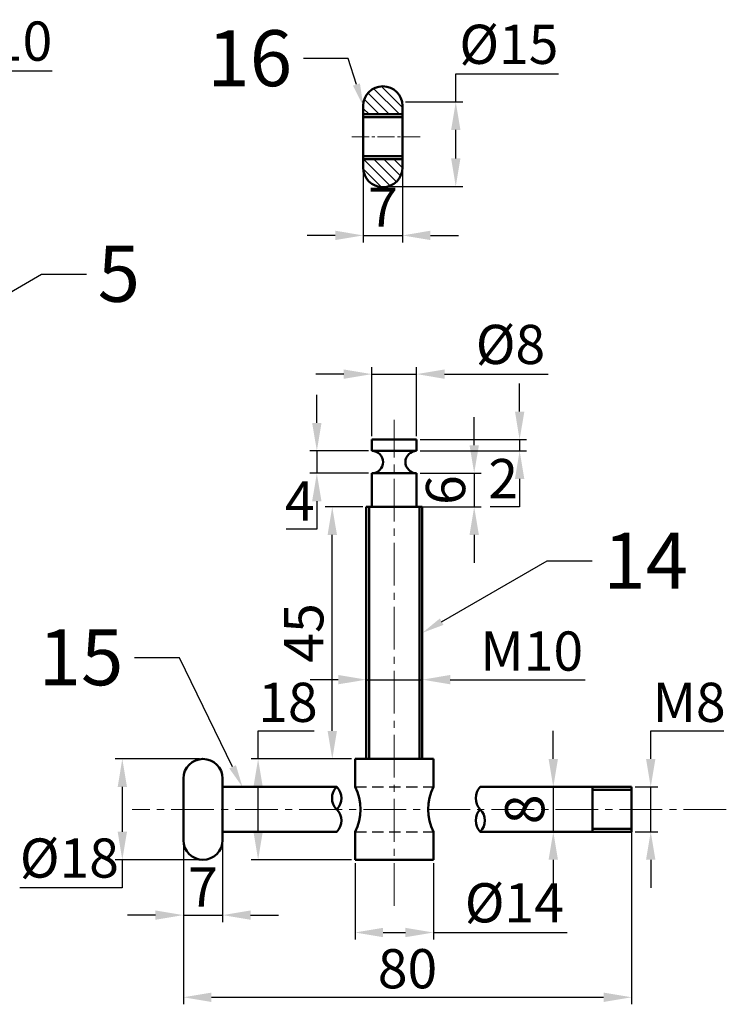
# Model space of a CAD drawing. Units: millimetres. Extents: x 434 to 1535, y -197 to 318.
# Tile 6 of 9: x 920 to 1046, y -7 to 168. Entities that reach past the tile are written whole.
import ezdxf
from ezdxf import colors
from ezdxf.entities.mleader import LeaderData, LeaderLine
from ezdxf.math import Vec2, Vec3

# ---------------------------------------------------------------- set-up
doc = ezdxf.new("R2010")
doc.units = ezdxf.units.MM
doc.header["$LTSCALE"] = 0.4
doc.linetypes.add('CENTER2', pattern=[28.575, 19.05, -3.175, 3.175, -3.175])
doc.linetypes.add('DASHED', pattern=[19.05, 12.7, -6.35])
for name, color, linetype, lineweight in [('M-CNTR', 1, 'CENTER2', 18), ('M-DIMS', 2, 'Continuous', 25), ('M-HATC', 8, 'Continuous', 18), ('M-HIDN', 6, 'DASHED', 25), ('M-OUTL', 7, 'Continuous', 50), ('M-TEXT', 3, 'Continuous', 25)]:
    doc.layers.add(name, color=color, linetype=linetype, lineweight=lineweight)
doc.styles.get("Standard").update_dxf_attribs({"font": 'arial.ttf'})
doc.dimstyles.new('ISO-25', dxfattribs={"dimtxt": 7, "dimasz": 5, "dimexe": 1.25, "dimexo": 0.625, "dimtad": 1, "dimtoh": 1, "dimdec": 0, "dimtxsty": 'Standard', "dimcen": 2.5, "dimadec": 0, "dimazin": 0, "dimtfac": 1, "dimtdec": 0, "dimtmove": 0, "dimatfit": 3, "dimfxl": 1, "dimarcsym": 0})

# ---------------------------------------------------------------- blocks, each defined once
blk = doc.blocks.new('*D61')
at = {"layer": 'Defpoints', "color": 0, "ltscale": 0.4, "transparency": 16777216}
for p in [(901.74, 149.22), (901.74, 139.22), (907.09, 139.22)]:
    blk.add_point(p, dxfattribs=at)
at = {"layer": 'M-DIMS', "color": 0, "lineweight": -2, "ltscale": 0.4, "transparency": 16777216}
for p, q in [((907.09, 154.22), (907.09, 159.22)), ((907.09, 159.22), (925.34, 159.22)), ((902.36, 149.22), (908.34, 149.22)), ((907.09, 139.22), (907.09, 149.22)), ((902.36, 139.22), (908.34, 139.22)), ((907.09, 134.22), (907.09, 129.22))]:
    blk.add_line(p, q, dxfattribs=at)
at = {"layer": 'M-DIMS', "color": 0, "ltscale": 0.4, "transparency": 16777216}
for points in [[(906.26, 154.22), (907.93, 154.22), (907.09, 149.22)], [(906.26, 134.22), (907.93, 134.22), (907.09, 139.22)]]:
    blk.add_solid(points, dxfattribs=at)
at = {"layer": 'M-DIMS', "color": 0, "ltscale": 0.4, "transparency": 16777216, "insert": (916.53, 163.61), "char_height": 7, "attachment_point": 5}
blk.add_mtext('%%C10', dxfattribs=at)
blk = doc.blocks.new('*U76')
at = {"layer": 'M-CNTR', "color": 0, "transparency": 16777216}
blk.add_line((0, -17.2), (0, 69.52), dxfattribs=at)
blk = doc.blocks.new('*U77')
at = {"layer": 'M-CNTR', "color": 0, "transparency": 16777216}
blk.add_line((59.26, 0), (-46.77, 0), dxfattribs=at)
blk = doc.blocks.new('*D78')
at = {"layer": 'Defpoints', "color": 0, "ltscale": 0.4, "transparency": 16777216}
for p in [(979.4, 18.37), (993.4, 18.37), (993.4, 5.38)]:
    blk.add_point(p, dxfattribs=at)
at = {"layer": 'M-DIMS', "color": 0, "lineweight": -2, "ltscale": 0.4, "transparency": 16777216}
for p, q in [((979.4, 17.75), (979.4, 4.13)), ((993.4, 17.75), (993.4, 4.13)), ((984.4, 5.38), (988.4, 5.38)), ((993.4, 5.38), (1017.27, 5.38))]:
    blk.add_line(p, q, dxfattribs=at)
at = {"layer": 'M-DIMS', "color": 0, "ltscale": 0.4, "transparency": 16777216}
for points in [[(984.4, 6.22), (984.4, 4.55), (979.4, 5.38)], [(988.4, 6.22), (988.4, 4.55), (993.4, 5.38)]]:
    blk.add_solid(points, dxfattribs=at)
at = {"layer": 'M-DIMS', "color": 0, "ltscale": 0.4, "transparency": 16777216, "insert": (1007.83, 9.78), "char_height": 7, "attachment_point": 5}
blk.add_mtext('%%C14', dxfattribs=at)
blk = doc.blocks.new('*D79')
at = {"layer": 'Defpoints', "color": 0, "ltscale": 0.4, "transparency": 16777216}
for p in [(948.77, 27.37), (1028.77, 27.37), (1028.77, -6.18)]:
    blk.add_point(p, dxfattribs=at)
at = {"layer": 'M-DIMS', "color": 0, "lineweight": -2, "ltscale": 0.4, "transparency": 16777216}
for p, q in [((948.77, 26.75), (948.77, -7.43)), ((1028.77, 26.75), (1028.77, -7.43)), ((953.77, -6.18), (1023.77, -6.18))]:
    blk.add_line(p, q, dxfattribs=at)
at = {"layer": 'M-DIMS', "color": 0, "ltscale": 0.4, "transparency": 16777216}
for points in [[(953.77, -5.35), (953.77, -7.02), (948.77, -6.18)], [(1023.77, -5.35), (1023.77, -7.02), (1028.77, -6.18)]]:
    blk.add_solid(points, dxfattribs=at)
at = {"layer": 'M-DIMS', "color": 0, "ltscale": 0.4, "transparency": 16777216, "insert": (988.77, -1.99), "char_height": 7, "attachment_point": 5}
blk.add_mtext('80', dxfattribs=at)
blk = doc.blocks.new('*D82')
at = {"layer": 'Defpoints', "color": 0, "ltscale": 0.4, "transparency": 16777216}
for p in [(1028.77, 31.37), (1028.77, 23.37), (1032.18, 23.37)]:
    blk.add_point(p, dxfattribs=at)
at = {"layer": 'M-DIMS', "color": 0, "lineweight": -2, "ltscale": 0.4, "transparency": 16777216}
for p, q in [((1032.18, 36.37), (1032.18, 41.37)), ((1032.18, 41.37), (1045.23, 41.37)), ((1029.4, 31.37), (1033.43, 31.37)), ((1032.18, 23.37), (1032.18, 31.37)), ((1029.4, 23.37), (1033.43, 23.37)), ((1032.18, 18.37), (1032.18, 13.37))]:
    blk.add_line(p, q, dxfattribs=at)
at = {"layer": 'M-DIMS', "color": 0, "ltscale": 0.4, "transparency": 16777216}
for points in [[(1031.34, 36.37), (1033.01, 36.37), (1032.18, 31.37)], [(1031.34, 18.37), (1033.01, 18.37), (1032.18, 23.37)]]:
    blk.add_solid(points, dxfattribs=at)
at = {"layer": 'M-DIMS', "color": 0, "ltscale": 0.4, "transparency": 16777216, "insert": (1039.02, 45.57), "char_height": 7, "attachment_point": 5}
blk.add_mtext('M8', dxfattribs=at)
blk = doc.blocks.new('*D83')
at = {"layer": 'Defpoints', "color": 0, "ltscale": 0.4, "transparency": 16777216}
for p in [(952.27, 36.37), (937.87, 18.37), (952.27, 18.37)]:
    blk.add_point(p, dxfattribs=at)
at = {"layer": 'M-DIMS', "color": 0, "lineweight": -2, "ltscale": 0.4, "transparency": 16777216}
for p, q in [((951.65, 36.37), (936.62, 36.37)), ((937.87, 31.37), (937.87, 23.37)), ((951.65, 18.37), (936.62, 18.37)), ((937.87, 18.37), (937.87, 13.37)), ((937.87, 13.37), (919.59, 13.37))]:
    blk.add_line(p, q, dxfattribs=at)
at = {"layer": 'M-DIMS', "color": 0, "ltscale": 0.4, "transparency": 16777216}
for points in [[(937.04, 31.37), (938.71, 31.37), (937.87, 36.37)], [(937.04, 23.37), (938.71, 23.37), (937.87, 18.37)]]:
    blk.add_solid(points, dxfattribs=at)
at = {"layer": 'M-DIMS', "color": 0, "ltscale": 0.4, "transparency": 16777216, "insert": (928.42, 17.77), "char_height": 7, "attachment_point": 5}
blk.add_mtext('%%C18', dxfattribs=at)
blk = doc.blocks.new('*D84')
at = {"layer": 'Defpoints', "color": 0, "ltscale": 0.4, "transparency": 16777216}
for p in [(948.77, 27.37), (955.77, 27.37), (955.77, 8.49)]:
    blk.add_point(p, dxfattribs=at)
at = {"layer": 'M-DIMS', "color": 0, "lineweight": -2, "ltscale": 0.4, "transparency": 16777216}
for p, q in [((948.77, 26.75), (948.77, 7.24)), ((955.77, 26.75), (955.77, 7.24)), ((943.77, 8.49), (938.77, 8.49)), ((948.77, 8.49), (955.77, 8.49)), ((960.77, 8.49), (965.77, 8.49))]:
    blk.add_line(p, q, dxfattribs=at)
at = {"layer": 'M-DIMS', "color": 0, "ltscale": 0.4, "transparency": 16777216}
for points in [[(943.77, 9.32), (943.77, 7.66), (948.77, 8.49)], [(960.77, 9.32), (960.77, 7.66), (955.77, 8.49)]]:
    blk.add_solid(points, dxfattribs=at)
at = {"layer": 'M-DIMS', "color": 0, "ltscale": 0.4, "transparency": 16777216, "insert": (952.27, 12.61), "char_height": 7, "attachment_point": 5}
blk.add_mtext('7', dxfattribs=at)
blk = doc.blocks.new('*D85')
at = {"layer": 'Defpoints', "color": 0, "ltscale": 0.4, "transparency": 16777216}
for p in [(962.11, 36.37), (979.4, 36.37), (979.4, 18.37)]:
    blk.add_point(p, dxfattribs=at)
at = {"layer": 'M-DIMS', "color": 0, "lineweight": -2, "ltscale": 0.4, "transparency": 16777216}
for p, q in [((962.11, 36.37), (962.11, 41.37)), ((962.11, 41.37), (972.12, 41.37)), ((978.78, 36.37), (960.86, 36.37)), ((962.11, 23.37), (962.11, 31.37)), ((978.78, 18.37), (960.86, 18.37))]:
    blk.add_line(p, q, dxfattribs=at)
at = {"layer": 'M-DIMS', "color": 0, "ltscale": 0.4, "transparency": 16777216}
for points in [[(961.28, 31.37), (962.94, 31.37), (962.11, 36.37)], [(961.28, 23.37), (962.94, 23.37), (962.11, 18.37)]]:
    blk.add_solid(points, dxfattribs=at)
at = {"layer": 'M-DIMS', "color": 0, "ltscale": 0.4, "transparency": 16777216, "insert": (967.43, 45.57), "char_height": 7, "attachment_point": 5}
blk.add_mtext('18', dxfattribs=at)
blk = doc.blocks.new('*D86')
at = {"layer": 'Defpoints', "color": 0, "ltscale": 0.4, "transparency": 16777216}
for p in [(975.34, 81.37), (981.4, 81.37), (979.4, 36.37)]:
    blk.add_point(p, dxfattribs=at)
at = {"layer": 'M-DIMS', "color": 0, "lineweight": -2, "ltscale": 0.4, "transparency": 16777216}
for p, q in [((980.78, 81.37), (974.09, 81.37)), ((975.34, 41.37), (975.34, 76.37)), ((978.78, 36.37), (974.09, 36.37))]:
    blk.add_line(p, q, dxfattribs=at)
at = {"layer": 'M-DIMS', "color": 0, "ltscale": 0.4, "transparency": 16777216}
for points in [[(974.51, 76.37), (976.18, 76.37), (975.34, 81.37)], [(974.51, 41.37), (976.18, 41.37), (975.34, 36.37)]]:
    blk.add_solid(points, dxfattribs=at)
at = {"layer": 'M-DIMS', "color": 0, "ltscale": 0.4, "transparency": 16777216, "insert": (971.16, 58.87), "char_height": 7, "attachment_point": 5, "rotation": 90}
blk.add_mtext('45', dxfattribs=at)
blk = doc.blocks.new('*D87')
at = {"layer": 'Defpoints', "color": 0, "ltscale": 0.4, "transparency": 16777216}
for p in [(990.4, 87.37), (990.4, 81.37), (1000.67, 81.37)]:
    blk.add_point(p, dxfattribs=at)
at = {"layer": 'M-DIMS', "color": 0, "lineweight": -2, "ltscale": 0.4, "transparency": 16777216}
for p, q in [((1000.67, 92.37), (1000.67, 97.37)), ((991.03, 87.37), (1001.92, 87.37)), ((1000.67, 87.37), (1000.67, 81.37)), ((991.03, 81.37), (1001.92, 81.37)), ((1000.67, 76.37), (1000.67, 71.37))]:
    blk.add_line(p, q, dxfattribs=at)
at = {"layer": 'M-DIMS', "color": 0, "ltscale": 0.4, "transparency": 16777216}
for points in [[(999.84, 92.37), (1001.51, 92.37), (1000.67, 87.37)], [(999.84, 76.37), (1001.51, 76.37), (1000.67, 81.37)]]:
    blk.add_solid(points, dxfattribs=at)
at = {"layer": 'M-DIMS', "color": 0, "ltscale": 0.4, "transparency": 16777216, "insert": (996.47, 84.37), "char_height": 7, "attachment_point": 5, "rotation": 90}
blk.add_mtext('6', dxfattribs=at)
blk = doc.blocks.new('*D88')
at = {"layer": 'Defpoints', "color": 0, "ltscale": 0.4, "transparency": 16777216}
for p in [(982.4, 91.37), (972.59, 87.37), (982.4, 87.37)]:
    blk.add_point(p, dxfattribs=at)
at = {"layer": 'M-DIMS', "color": 0, "lineweight": -2, "ltscale": 0.4, "transparency": 16777216}
for p, q in [((972.59, 96.37), (972.59, 101.37)), ((981.78, 91.37), (971.34, 91.37)), ((972.59, 91.37), (972.59, 87.37)), ((981.78, 87.37), (971.34, 87.37)), ((972.59, 82.37), (972.59, 77.37)), ((972.59, 77.37), (967.12, 77.37))]:
    blk.add_line(p, q, dxfattribs=at)
at = {"layer": 'M-DIMS', "color": 0, "ltscale": 0.4, "transparency": 16777216}
for points in [[(971.75, 96.37), (973.42, 96.37), (972.59, 91.37)], [(971.75, 82.37), (973.42, 82.37), (972.59, 87.37)]]:
    blk.add_solid(points, dxfattribs=at)
at = {"layer": 'M-DIMS', "color": 0, "ltscale": 0.4, "transparency": 16777216, "insert": (969.54, 81.5), "char_height": 7, "attachment_point": 5}
blk.add_mtext('4', dxfattribs=at)
blk = doc.blocks.new('*D89')
at = {"layer": 'Defpoints', "color": 0, "ltscale": 0.4, "transparency": 16777216}
for p in [(990.4, 93.37), (990.4, 91.37), (1008.78, 91.37)]:
    blk.add_point(p, dxfattribs=at)
at = {"layer": 'M-DIMS', "color": 0, "lineweight": -2, "ltscale": 0.4, "transparency": 16777216}
for p, q in [((1008.78, 98.37), (1008.78, 103.37)), ((991.03, 93.37), (1010.03, 93.37)), ((1008.78, 93.37), (1008.78, 91.37)), ((991.03, 91.37), (1010.03, 91.37)), ((1008.78, 86.37), (1008.78, 81.37)), ((1008.78, 81.37), (1003.52, 81.37))]:
    blk.add_line(p, q, dxfattribs=at)
at = {"layer": 'M-DIMS', "color": 0, "ltscale": 0.4, "transparency": 16777216}
for points in [[(1007.95, 98.37), (1009.62, 98.37), (1008.78, 93.37)], [(1007.95, 86.37), (1009.62, 86.37), (1008.78, 91.37)]]:
    blk.add_solid(points, dxfattribs=at)
at = {"layer": 'M-DIMS', "color": 0, "ltscale": 0.4, "transparency": 16777216, "insert": (1005.84, 85.51), "char_height": 7, "attachment_point": 5}
blk.add_mtext('2', dxfattribs=at)
blk = doc.blocks.new('*D90')
at = {"layer": 'Defpoints', "color": 0, "ltscale": 0.4, "transparency": 16777216}
for p in [(990.4, 105.07), (982.4, 93.37), (990.4, 93.37)]:
    blk.add_point(p, dxfattribs=at)
at = {"layer": 'M-DIMS', "color": 0, "lineweight": -2, "ltscale": 0.4, "transparency": 16777216}
for p, q in [((982.4, 94), (982.4, 106.32)), ((990.4, 94), (990.4, 106.32)), ((977.4, 105.07), (972.4, 105.07)), ((982.4, 105.07), (990.4, 105.07)), ((995.4, 105.07), (1013.87, 105.07))]:
    blk.add_line(p, q, dxfattribs=at)
at = {"layer": 'M-DIMS', "color": 0, "ltscale": 0.4, "transparency": 16777216}
for points in [[(977.4, 105.9), (977.4, 104.23), (982.4, 105.07)], [(995.4, 105.9), (995.4, 104.23), (990.4, 105.07)]]:
    blk.add_solid(points, dxfattribs=at)
at = {"layer": 'M-DIMS', "color": 0, "ltscale": 0.4, "transparency": 16777216, "insert": (1007.14, 109.46), "char_height": 7, "attachment_point": 5}
blk.add_mtext('%%C8', dxfattribs=at)
blk = doc.blocks.new('*D91')
at = {"layer": 'Defpoints', "color": 0, "ltscale": 0.4, "transparency": 16777216}
for p in [(991.4, 50.52), (981.4, 48.18), (991.4, 48.18)]:
    blk.add_point(p, dxfattribs=at)
at = {"layer": 'M-DIMS', "color": 0, "lineweight": -2, "ltscale": 0.4, "transparency": 16777216}
for p, q in [((981.4, 48.8), (981.4, 51.77)), ((991.4, 48.8), (991.4, 51.77)), ((976.4, 50.52), (971.4, 50.52)), ((981.4, 50.52), (991.4, 50.52)), ((996.4, 50.52), (1020.48, 50.52))]:
    blk.add_line(p, q, dxfattribs=at)
at = {"layer": 'M-DIMS', "color": 0, "ltscale": 0.4, "transparency": 16777216}
for points in [[(976.4, 51.36), (976.4, 49.69), (981.4, 50.52)], [(996.4, 51.36), (996.4, 49.69), (991.4, 50.52)]]:
    blk.add_solid(points, dxfattribs=at)
at = {"layer": 'M-DIMS', "color": 0, "ltscale": 0.4, "transparency": 16777216, "insert": (1010.94, 54.72), "char_height": 7, "attachment_point": 5}
blk.add_mtext('M10', dxfattribs=at)
blk = doc.blocks.new('*D92')
at = {"layer": 'Defpoints', "color": 0, "ltscale": 0.4, "transparency": 16777216}
for p in [(1012.69, 31.37), (1012.69, 23.37), (1014.79, 23.37)]:
    blk.add_point(p, dxfattribs=at)
at = {"layer": 'M-DIMS', "color": 0, "lineweight": -2, "ltscale": 0.4, "transparency": 16777216}
for p, q in [((1014.79, 36.37), (1014.79, 41.37)), ((1013.32, 31.37), (1016.04, 31.37)), ((1014.79, 31.37), (1014.79, 23.37)), ((1013.32, 23.37), (1016.04, 23.37)), ((1014.79, 18.37), (1014.79, 13.37))]:
    blk.add_line(p, q, dxfattribs=at)
at = {"layer": 'M-DIMS', "color": 0, "ltscale": 0.4, "transparency": 16777216}
for points in [[(1013.95, 36.37), (1015.62, 36.37), (1014.79, 31.37)], [(1013.95, 18.37), (1015.62, 18.37), (1014.79, 23.37)]]:
    blk.add_solid(points, dxfattribs=at)
at = {"layer": 'M-DIMS', "color": 0, "ltscale": 0.4, "transparency": 16777216, "insert": (1010.59, 27.37), "char_height": 7, "attachment_point": 5, "rotation": 90}
blk.add_mtext('8', dxfattribs=at)
blk = doc.blocks.new('*D93')
at = {"layer": 'Defpoints', "color": 0, "ltscale": 0.4, "transparency": 16777216}
for p in [(987.79, 153.65), (983.38, 138.59), (997.38, 138.59)]:
    blk.add_point(p, dxfattribs=at)
at = {"layer": 'M-DIMS', "color": 0, "lineweight": -2, "ltscale": 0.4, "transparency": 16777216}
for p, q in [((997.38, 153.65), (997.38, 158.65)), ((997.38, 158.65), (1015.7, 158.65)), ((988.42, 153.65), (998.63, 153.65)), ((997.38, 143.59), (997.38, 148.65)), ((984.01, 138.59), (998.63, 138.59))]:
    blk.add_line(p, q, dxfattribs=at)
at = {"layer": 'M-DIMS', "color": 0, "ltscale": 0.4, "transparency": 16777216}
for points in [[(996.55, 148.65), (998.22, 148.65), (997.38, 153.65)], [(996.55, 143.59), (998.22, 143.59), (997.38, 138.59)]]:
    blk.add_solid(points, dxfattribs=at)
at = {"layer": 'M-DIMS', "color": 0, "ltscale": 0.4, "transparency": 16777216, "insert": (1006.86, 163.04), "char_height": 7, "attachment_point": 5}
blk.add_mtext('%%C15', dxfattribs=at)
blk = doc.blocks.new('*D94')
at = {"layer": 'Defpoints', "color": 0, "ltscale": 0.4, "transparency": 16777216}
for p in [(980.87, 145.12), (987.87, 145.12), (987.87, 129.83)]:
    blk.add_point(p, dxfattribs=at)
at = {"layer": 'M-DIMS', "color": 0, "lineweight": -2, "ltscale": 0.4, "transparency": 16777216}
for p, q in [((980.87, 144.49), (980.87, 128.58)), ((987.87, 144.49), (987.87, 128.58)), ((975.87, 129.83), (970.87, 129.83)), ((980.87, 129.83), (987.87, 129.83)), ((992.87, 129.83), (997.87, 129.83))]:
    blk.add_line(p, q, dxfattribs=at)
at = {"layer": 'M-DIMS', "color": 0, "ltscale": 0.4, "transparency": 16777216}
for points in [[(975.87, 130.67), (975.87, 129), (980.87, 129.83)], [(992.87, 130.67), (992.87, 129), (987.87, 129.83)]]:
    blk.add_solid(points, dxfattribs=at)
at = {"layer": 'M-DIMS', "color": 0, "ltscale": 0.4, "transparency": 16777216, "insert": (984.37, 133.96), "char_height": 7, "attachment_point": 5}
blk.add_mtext('7', dxfattribs=at)
blk = doc.blocks.new('HANDLE-GRIP')
at = {"ltscale": 0.4}
for p, q in [((0, 14.5), (0, 3.5)), ((7, 3.5), (7, 14.5))]:
    blk.add_line(p, q, dxfattribs=at)
for centre, start, end in [((3.5, 14.5), 0, 180), ((3.5, 3.5), 180, 0)]:
    blk.add_arc(centre, 3.5, start, end, dxfattribs=at)

msp = doc.modelspace()

# ---------------------------------------------------------------- hatches: boundary and pattern name
at = {"layer": 'M-HATC', "ltscale": 0.4}
h = msp.add_hatch(dxfattribs=at)
h.set_pattern_fill('ANSI31', color=256, scale=0.4, angle=90)
h.set_pattern_definition([(135, (-240.3132, 385.8592), (-0.8980256, -0.8980256), [])])
h.paths.add_polyline_path([(987.87, 152.95, 1), (980.87, 152.95), (980.87, 151.45), (987.87, 151.45)])
h.paths.add_polyline_path([(987.87, 141.95), (987.87, 143.45), (980.87, 143.45), (980.87, 141.95, 1)])

# ---------------------------------------------------------------- linework, layer by layer
at = {"layer": 'M-CNTR', "ltscale": 0.4}
msp.add_line((991.05, 147.45), (978.76, 147.45), dxfattribs=at)
at = {"layer": 'M-HIDN', "ltscale": 0.4}
for p, q in [((979.4, 31.37), (993.4, 31.37)), ((979.4, 23.37), (993.4, 23.37))]:
    msp.add_line(p, q, dxfattribs=at)
at = {"layer": 'M-OUTL', "ltscale": 0.4}
for p, q in [((987.87, 151.45), (980.87, 151.45)), ((987.87, 150.95), (980.87, 150.95)), ((987.87, 143.95), (980.87, 143.95)), ((987.87, 143.45), (980.87, 143.45)), ((982.4, 91.37), (982.4, 93.37)), ((982.4, 93.37), (990.4, 93.37)), ((990.4, 93.37), (990.4, 91.37)), ((990.4, 91.37), (982.4, 91.37)), ((990.4, 87.37), (982.4, 87.37)), ((982.4, 87.37), (982.4, 81.37)), ((990.4, 81.37), (990.4, 87.37)), ((991.4, 81.37), (981.4, 81.37)), ((981.4, 36.37), (981.4, 81.37)), ((981.9, 36.37), (981.9, 81.37)), ((990.9, 36.37), (990.9, 81.37)), ((991.4, 36.37), (991.4, 81.37)), ((979.4, 36.37), (979.4, 31.37)), ((993.4, 36.37), (979.4, 36.37)), ((993.4, 31.37), (993.4, 36.37)), ((976.13, 31.37), (955.77, 31.37)), ((1028.77, 31.37), (1001.76, 31.37)), ((1021.77, 23.37), (1021.77, 31.37)), ((1021.77, 30.87), (1028.77, 30.87)), ((1028.77, 23.37), (1028.77, 31.37)), ((976.13, 23.37), (955.77, 23.37)), ((979.4, 23.37), (979.4, 18.37)), ((993.4, 18.37), (993.4, 23.37)), ((1028.77, 23.37), (1001.76, 23.37)), ((1021.77, 23.87), (1028.77, 23.87)), ((979.4, 18.37), (993.4, 18.37))]:
    msp.add_line(p, q, dxfattribs=at)
for centre, radius, start, end in [((982.4, 89.37), 2, 270, 90), ((990.4, 89.37), 2, 90, 270), ((978.14, 29.37), 2.84, 135.1658, 224.8342), ((974.12, 29.37), 2.84, 315.1658, 44.8342), ((971.55, 27.37), 8.81, 332.9936, 27.0064), ((1001.25, 27.37), 8.81, 152.9936, 207.0064), ((1003.82, 29.37), 2.87, 135.7983, 224.2017), ((974.12, 25.37), 2.84, 315.1658, 44.8342), ((1003.82, 25.37), 2.87, 135.7983, 224.2017), ((999.71, 25.37), 2.87, 315.7983, 44.2017)]:
    msp.add_arc(centre, radius, start, end, dxfattribs=at)

# ---------------------------------------------------------------- block references
at = {"layer": 'M-CNTR'}
for name in ['*U76', '*U77']:
    msp.add_blockref(name, (986.4, 27.37), dxfattribs=at)
at = {"layer": 'M-OUTL', "rotation": 180}
msp.add_blockref('HANDLE-GRIP', (987.87, 156.45), dxfattribs=at)
at = {"layer": 'M-OUTL'}
msp.add_blockref('HANDLE-GRIP', (948.77, 18.37), dxfattribs=at)

# ---------------------------------------------------------------- dimensions: what is measured, and where the dimension line sits
at = {"layer": 'M-DIMS', "ltscale": 0.4}
for base, p1, p2, text, picture, middle in [((907.09, 139.22), (901.74, 149.22), (901.74, 139.22), '%%C<>', '*D61', (916.53, 159.22)), ((997.38, 138.59), (987.79, 153.65), (983.38, 138.59), '%%C<>', '*D93', (1006.86, 158.65)), ((1032.18, 23.37), (1028.77, 31.37), (1028.77, 23.37), 'M<>', '*D82', (1039.02, 41.37))]:
    dim = msp.add_linear_dim(base=base, p1=p1, p2=p2, angle=90, text=text, dimstyle='ISO-25', override={"dimclrd": 0, "dimclre": 0, "dimclrt": 0}, dxfattribs=at)
    dim.commit()
    dim.dimension.update_dxf_attribs({"geometry": picture, "text_midpoint": middle, "dimtype": 160})
for base, p1, p2, picture, middle in [((987.87, 129.83), (980.87, 145.12), (987.87, 145.12), '*D94', (984.37, 133.96)), ((955.77, 8.49), (948.77, 27.37), (955.77, 27.37), '*D84', (952.27, 12.61)), ((1028.77, -6.18), (948.77, 27.37), (1028.77, 27.37), '*D79', (988.77, -1.99))]:
    dim = msp.add_linear_dim(base=base, p1=p1, p2=p2, dimstyle='ISO-25', override={"dimclrd": 0, "dimclre": 0, "dimclrt": 0}, dxfattribs=at)
    dim.commit()
    dim.dimension.update_dxf_attribs({"geometry": picture, "text_midpoint": middle})
for base, p1, p2, text, picture, middle in [((990.4, 105.07), (982.4, 93.37), (990.4, 93.37), '%%C<>', '*D90', (1007.14, 109.46)), ((991.4, 50.52), (981.4, 48.18), (991.4, 48.18), 'M<>', '*D91', (1010.94, 54.72)), ((993.4, 5.38), (979.4, 18.37), (993.4, 18.37), '%%C<>', '*D78', (1007.83, 9.78))]:
    dim = msp.add_linear_dim(base=base, p1=p1, p2=p2, text=text, dimstyle='ISO-25', override={"dimclrd": 0, "dimclre": 0, "dimclrt": 0}, dxfattribs=at)
    dim.commit()
    dim.dimension.update_dxf_attribs({"geometry": picture, "text_midpoint": middle})
for base, p1, p2, picture, middle in [((1008.78, 91.37), (990.4, 93.37), (990.4, 91.37), '*D89', (1005.84, 85.51)), ((972.59, 87.37), (982.4, 91.37), (982.4, 87.37), '*D88', (969.54, 81.5)), ((1000.67, 81.37), (990.4, 87.37), (990.4, 81.37), '*D87', (996.47, 84.37)), ((975.34, 81.37), (979.4, 36.37), (981.4, 81.37), '*D86', (971.16, 58.87)), ((1014.79, 23.37), (1012.69, 31.37), (1012.69, 23.37), '*D92', (1010.59, 27.37))]:
    dim = msp.add_linear_dim(base=base, p1=p1, p2=p2, angle=90, dimstyle='ISO-25', override={"dimclrd": 0, "dimclre": 0, "dimclrt": 0}, dxfattribs=at)
    dim.commit()
    dim.dimension.update_dxf_attribs({"geometry": picture, "text_midpoint": middle})
dim = msp.add_linear_dim(base=(962.11, 36.37), p1=(979.4, 18.37), p2=(979.4, 36.37), angle=90, dimstyle='ISO-25', override={"dimclrd": 0, "dimclre": 0, "dimclrt": 0}, dxfattribs=at)
dim.commit()
dim.dimension.update_dxf_attribs({"geometry": '*D85', "text_midpoint": (967.43, 41.37), "dimtype": 160})
dim = msp.add_linear_dim(base=(937.87, 18.37), p1=(952.27, 36.37), p2=(952.27, 18.37), angle=90, text='%%C<>', dimstyle='ISO-25', override={"dimclrd": 0, "dimclre": 0, "dimclrt": 0}, dxfattribs=at)
dim.commit()
dim.dimension.update_dxf_attribs({"geometry": '*D83', "text_midpoint": (928.42, 17.77)})

# ---------------------------------------------------------------- leaders
at = {"layer": 'M-TEXT', "ltscale": 0.4}
ml = msp.add_multileader_mtext('Standard', dxfattribs=at)
ml.set_content('16', color=256)
ml.set_leader_properties()
ml.build(insert=Vec2(0, 0))
ctx = ml.context
ctx.base_point, ctx.char_height, ctx.plane_origin = Vec3(952.8, 161.39), 10, Vec3(980.87, 152.95)
ctx.text_align_type = 2
notes = []
notes.append((ctx, [(0, (1, 1, 0), (978.18, 161.39), (-1, 0), 8, [(0, [(980.87, 152.95)], 0, [])])]))
ctx.mtext.insert, ctx.mtext.alignment, ctx.mtext.flow_direction = Vec3(968.18, 166.47), 3, 5
ml = msp.add_multileader_mtext('Standard', dxfattribs=at)
ml.set_content('5', color=256)
ml.set_leader_properties()
ml.build(insert=Vec2(0, 0))
ctx = ml.context
ctx.base_point, ctx.char_height, ctx.plane_origin = Vec3(931.47, 122.89), 10, Vec3(898.24, 108.33)
notes.append((ctx, [(0, (1, 1, 0), (923.47, 122.89), (1, 0), 8, [(0, [(898.24, 108.33)], 0, [])])]))
ctx.mtext.insert, ctx.mtext.flow_direction = Vec3(933.47, 127.98), 5
ml = msp.add_multileader_mtext('Standard', dxfattribs=at)
ml.set_content('14', color=256)
ml.set_leader_properties()
ml.build(insert=Vec2(0, 0))
ctx = ml.context
ctx.base_point, ctx.char_height, ctx.plane_origin = Vec3(1021.71, 71.75), 10, Vec3(991.4, 58.87)
notes.append((ctx, [(0, (1, 1, 0), (1013.71, 71.75), (1, 0), 8, [(0, [(991.4, 58.87)], 0, [])])]))
ctx.mtext.insert, ctx.mtext.flow_direction = Vec3(1023.71, 76.75), 5
ml = msp.add_multileader_mtext('Standard', dxfattribs=at)
ml.set_content('15', color=256)
ml.set_leader_properties()
ml.build(insert=Vec2(0, 0))
ctx = ml.context
ctx.base_point, ctx.char_height, ctx.plane_origin = Vec3(922.61, 54.44), 10, Vec3(959.31, 31.37)
ctx.text_align_type = 2
notes.append((ctx, [(0, (1, 1, 0), (948.07, 54.44), (-1, 0), 8, [(0, [(959.31, 31.37)], 0, [])])]))
ctx.mtext.insert, ctx.mtext.alignment, ctx.mtext.flow_direction = Vec3(938.07, 59.52), 3, 5
for ctx, leaders in notes:
    for number, flags, end, landing, length, lines in leaders:
        leader = LeaderData()
        leader.index, (leader.has_last_leader_line, leader.has_dogleg_vector, leader.attachment_direction) = number, flags
        leader.last_leader_point, leader.dogleg_vector, leader.dogleg_length = Vec3(end), Vec3(landing), length
        for number, points, colour, breaks in lines:
            line = LeaderLine()
            line.index, line.vertices, line.color, line.breaks = number, Vec3.list(points), colors.encode_raw_color(colour), breaks
            leader.lines.append(line)
        ctx.leaders.append(leader)

doc.saveas('drawing.dxf')
